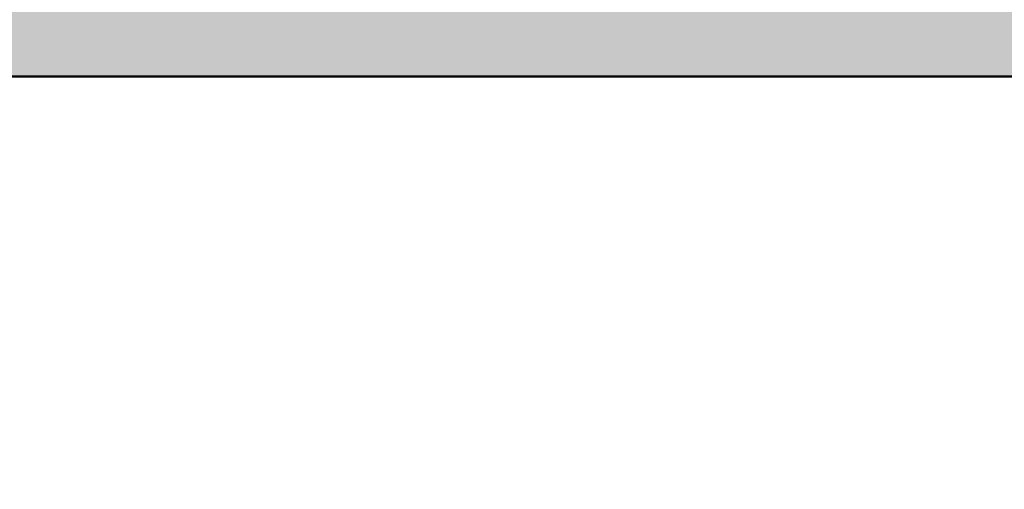
# Model space of a CAD drawing. Units: inches. Extents: x -7 to 1228, y -146 to 1091.
# Tile 65 of 88: x 656 to 745, y 531 to 573. Entities that reach past the tile are written whole.
import ezdxf

# ---------------------------------------------------------------- set-up
doc = ezdxf.new("R2010")
doc.units = ezdxf.units.IN
doc.layers.add('A-WALL', color=7, linetype='Continuous', lineweight=50)
doc.layers.add('A-WALL-PATT', color=251, linetype='Continuous', lineweight=13)

msp = doc.modelspace()

# ---------------------------------------------------------------- hatches: boundary and pattern name
at = {"layer": 'A-WALL-PATT'}
h = msp.add_hatch(color=256, dxfattribs=at)
h.dxf.hatch_style = 1
h.paths.add_polyline_path([(69, 568), (60, 568), (60, 493), (63.289, 493), (69, 493)])
h.paths.add_polyline_path([(69, 662.405), (60, 662.405), (60, 586), (69, 586)], flags=17)
h.paths.add_polyline_path([(69, 723), (184, 723), (184, 734), (179, 734), (179, 728), (69, 728), (69, 741.623), (60, 741.623), (60, 698.405), (69, 698.405)], flags=17)
h.paths.add_polyline_path([(69, 782), (231, 782), (231, 728), (231, 723), (231, 586), (236, 586), (236, 787), (69, 787), (69, 800.126), (60, 800.126), (60, 765.623), (69, 765.623)])
h.paths.add_polyline_path([(184, 842), (189, 842), (189, 848), (173, 848), (173, 842), (179, 842), (179, 787), (184, 787)])
h.paths.add_polyline_path([(118.22, 69), (69, 69), (69, 60), (118.22, 60)])
h.paths.add_polyline_path([(227, 69), (154.22, 69), (154.22, 60), (227, 60)])
h.paths.add_polyline_path([(236, 60), (232.711, 60), (227, 60), (227, 36), (236, 36)])
h.paths.add_polyline_path([(389, 60), (380, 60), (380, 36), (389, 36)])
h.paths.add_polyline_path([(384, 181), (380, 181), (380, 115), (380, 78), (384, 78)])
h.paths.add_polyline_path([(380, 115), (334.547, 115), (334.547, 109), (380, 109)])
h.paths.add_polyline_path([(274.547, 115), (236, 115), (236, 201), (232.711, 201), (231, 201), (231, 78), (236, 78), (236, 109), (274.547, 109)])
h.paths.add_polyline_path([(69, 123), (60, 123), (60, 78), (69, 78)])
h.paths.add_polyline_path([(69, 201), (60, 201), (60, 159), (69, 159)])
h.paths.add_polyline_path([(143, 219), (69, 219), (69, 213), (143, 213)], flags=17)
h.paths.add_polyline_path([(189, 219), (184, 219), (184, 274), (231, 274), (231, 219), (236, 219), (236, 279), (184, 279), (184, 297), (179, 297), (179, 279), (69, 279), (69, 290.912), (60, 290.912), (60, 262.179), (69, 262.179), (69, 274), (179, 274), (179, 219), (173, 219), (173, 213), (189, 213)])
h.paths.add_polyline_path([(69, 238.179), (60, 238.179), (60, 219), (69, 219)], flags=17)
h.paths.add_polyline_path([(69, 333), (60, 333), (60, 314.912), (69, 314.912), (69, 316.965)])
h.paths.add_polyline_path([(190, 338), (184, 338), (69, 338), (69, 333), (179, 333), (179, 327), (184, 327), (184, 333.021), (190, 333.046)])
h.paths.add_polyline_path([(69, 386.806), (60, 386.806), (60, 351), (69, 351)])
h.paths.add_polyline_path([(69, 475), (60, 475), (60, 422.806), (69, 422.806)])
h.paths.add_polyline_path([(236, 475), (231, 475), (231, 351.238), (236, 351.238)])
h.paths.add_polyline_path([(384, 475), (380, 475), (380, 362), (384, 362)])
h.paths.add_polyline_path([(547, 307), (439, 307), (439, 356), (445, 356), (445, 362), (433, 362), (433, 307), (380, 307), (380, 244), (380, 241), (384, 241), (384, 301), (433, 301), (433, 277), (439, 277), (439, 301), (547, 301)])
h.paths.add_polyline_path([(547, 241), (439, 241), (439, 247), (433, 247), (433, 235), (547, 235)])
h.paths.add_polyline_path([(450, 69), (440.286, 69), (424.889, 69), (389, 69), (389, 60), (450, 60)])
h.paths.add_polyline_path([(547, 69), (486, 69), (486, 60), (547, 60)])
h.paths.add_polyline_path([(556, 148.268), (547, 148.268), (547, 78), (556, 78)])
h.paths.add_polyline_path([(556, 223), (547, 223), (547, 195), (547, 184.268), (556, 184.268)])
h.paths.add_polyline_path([(556, 311.192), (547, 311.192), (547, 273.075), (556, 273.075)])
h.paths.add_polyline_path([(556, 344), (552.711, 344), (547, 344), (547, 335.192), (556, 335.192)])
h.paths.add_polyline_path([(556, 249.075), (547, 249.075), (547, 241), (556, 241)])
h.paths.add_polyline_path([(547, 362), (475, 362), (475, 356), (547, 356)], flags=0)
h.paths.add_polyline_path([(556, 399.621), (547, 399.621), (547, 362), (556, 362)])
h.paths.add_polyline_path([(556, 475), (547, 475), (547, 435.621), (556, 435.621)])
h.paths.add_polyline_path([(547, 493), (389, 493), (389, 487), (547, 487)])
h.paths.add_polyline_path([(380, 493), (278, 493), (278, 487), (380, 487)])
h.paths.add_polyline_path([(227, 493), (69, 493), (69, 487), (227, 487)])
h.paths.add_polyline_path([(643, 122.445), (634, 122.445), (634, 78), (643, 78)])
h.paths.add_polyline_path([(702.5, 69), (692.786, 69), (677.389, 69), (643, 69), (643, 60), (702.5, 60)])
h.paths.add_polyline_path([(798, 69), (738.5, 69), (738.5, 60), (798, 60)])
h.paths.add_polyline_path([(807, 60), (803.711, 60), (798, 60), (798, 36), (807, 36)])
h.paths.add_polyline_path([(807, 109), (846.751, 109), (846.751, 115), (807, 115), (807, 159), (802, 159), (802, 78), (807, 78)])
h.paths.add_polyline_path([(807, 201), (802, 201), (802, 195), (807, 195)])
h.paths.add_polyline_path([(643, 201), (634, 201), (634, 158.445), (643, 158.445)])
h.paths.add_polyline_path([(756, 225), (751, 225), (751, 219), (643, 219), (643, 213), (756, 213)])
h.paths.add_polyline_path([(643, 240.848), (634, 240.848), (634, 219), (643, 219)])
h.paths.add_polyline_path([(643, 274), (643, 288.629), (634, 288.629), (634, 264.848), (643, 264.848)])
h.paths.add_polyline_path([(802, 279), (756, 279), (756, 297), (751, 297), (751, 279), (643, 279), (643, 274), (751, 274), (751, 255), (756, 255), (756, 274), (802, 274)])
h.paths.add_polyline_path([(807, 333), (803.711, 333), (802, 333), (802, 279), (802, 274), (802, 219), (807, 219)])
h.paths.add_polyline_path([(956, 182), (951, 182), (951, 115), (906.751, 115), (906.751, 109), (951, 109), (951, 78), (956, 78)])
h.paths.add_polyline_path([(960, 60), (951, 60), (951, 36), (960, 36)])
h.paths.add_polyline_path([(1021, 69), (1005.781, 69), (960, 69), (960, 60), (1021, 60)])
h.paths.add_polyline_path([(956, 224), (951, 224), (951, 218), (956, 218)])
h.paths.add_polyline_path([(956, 302), (1004, 302), (1004, 278), (1010, 278), (1010, 302), (1118, 302), (1118, 290.809), (1127, 290.809), (1127, 326.968), (1118, 326.968), (1118, 320.966), (1118, 307), (1010, 307), (1010, 356), (1016, 356), (1016, 362), (1004, 362), (1004, 307), (951, 307), (951, 244), (951, 242), (954.289, 242), (956, 242)])
h.paths.add_polyline_path([(643, 333), (634, 333), (634, 312.629), (643, 312.629), (643, 316.965)])
h.paths.add_polyline_path([(756, 338), (643, 338), (643, 333), (751, 333), (751, 327), (756, 327)])
h.paths.add_polyline_path([(643, 388), (634, 388), (634, 351), (643, 351)])
h.paths.add_polyline_path([(807, 357), (802, 357), (802, 351), (807, 351)])
h.paths.add_polyline_path([(807, 475), (802, 475), (802, 393), (807, 393)])
h.paths.add_polyline_path([(643, 475), (634, 475), (634, 424), (643, 424)])
h.paths.add_polyline_path([(798, 493), (643, 493), (643, 487), (798, 487)])
h.paths.add_polyline_path([(634, 493), (556, 493), (556, 487), (634, 487)])
h.paths.add_polyline_path([(813, 493), (807, 493), (807, 487), (813, 487)])
h.paths.add_polyline_path([(951, 493), (849, 493), (849, 487), (951, 487)])
h.paths.add_polyline_path([(956, 484), (951, 484), (951, 374), (956, 374)])
h.paths.add_polyline_path([(1109, 493), (969, 493), (969, 487), (1109, 487)])
h.paths.add_polyline_path([(1127, 484), (1118, 484), (1118, 450.641), (1127, 450.641)])
h.paths.add_polyline_path([(1127, 414.641), (1118, 414.641), (1118, 365), (1127, 365)])
h.paths.add_polyline_path([(1109, 362), (1046, 362), (1046, 356), (1109, 356)], flags=17)
h.paths.add_polyline_path([(1127, 356), (1123.454, 356), (1118, 356), (1118, 350.968), (1127, 350.968)], flags=0)
h.paths.add_polyline_path([(1127, 266.809), (1118, 266.809), (1118, 262.361), (1118, 242), (1127, 242)], flags=17)
h.paths.add_polyline_path([(1118, 242), (1010, 242), (1010, 248), (1004, 248), (1004, 237), (1118, 237)])
h.paths.add_polyline_path([(1127, 224), (1118, 224), (1118, 170), (1127, 170)])
h.paths.add_polyline_path([(1127, 134), (1118, 134), (1118, 78), (1127, 78)])
h.paths.add_polyline_path([(1118, 69), (1057, 69), (1057, 60), (1118, 60)])
h.paths.add_polyline_path([(227, 571.546), (227, 574), (69, 574), (69, 568), (227, 568)])
h.paths.add_polyline_path([(380, 571.546), (380, 574), (278, 574), (278, 568), (380, 568)])
h.paths.add_polyline_path([(242, 574), (236, 574), (236, 568), (242, 568)])
h.paths.add_polyline_path([(547, 571.546), (547, 574), (389, 574), (389, 568), (547, 568)])
h.paths.add_polyline_path([(384, 733), (380, 733), (380, 586), (384, 586)])
h.paths.add_polyline_path([(556, 646), (634, 646), (634, 655), (547, 655), (547, 586), (556, 586)])
h.paths.add_polyline_path([(634, 574), (556, 574), (556, 568), (634, 568)])
h.paths.add_polyline_path([(643, 655), (634, 655), (634, 586), (643, 586)])
h.paths.add_polyline_path([(798, 574), (643, 574), (643, 568), (798, 568)])
h.paths.add_polyline_path([(643, 663.854), (634, 663.854), (634, 655), (643, 655)])
h.paths.add_polyline_path([(556, 676.967), (547, 676.967), (547, 655), (556, 655)])
h.paths.add_polyline_path([(556, 733), (547, 733), (547, 712.967), (556, 712.967)])
h.paths.add_polyline_path([(643, 710), (634, 710), (634, 699.854), (643, 699.854)])
h.paths.add_polyline_path([(807, 668), (802, 668), (802, 586), (807, 586)])
h.paths.add_polyline_path([(951, 574), (849, 574), (849, 568), (951, 568)])
h.paths.add_polyline_path([(956, 691), (951, 691), (951, 577), (956, 577)])
h.paths.add_polyline_path([(1109, 574), (969, 574), (969, 568), (1109, 568)])
h.paths.add_polyline_path([(1127, 643.403), (1118, 643.403), (1118, 577), (1127, 577)])
h.paths.add_polyline_path([(1127, 568), (1123.454, 568), (1118, 568), (1118, 493), (1127, 493)])
h.paths.add_polyline_path([(1127, 733), (1118, 733), (1118, 679.403), (1127, 679.403)])
h.paths.add_polyline_path([(1127, 777.348), (1118, 777.348), (1118, 770.035), (1118, 751), (1127, 751)], flags=17)
h.paths.add_polyline_path([(1118, 751), (1010, 751), (1010, 757), (1004, 757), (1004, 745), (1118, 745)])
h.paths.add_polyline_path([(956, 811), (1004, 811), (1004, 787), (1010, 787), (1010, 811), (1017.874, 811), (1017.874, 811.627, -0.414214), (1018.247, 812), (1031.978, 812, -0.414214), (1032.351, 811.627), (1032.351, 811), (1118, 811), (1118, 801.348), (1127, 801.348), (1127, 834.685), (1118, 834.685), (1118, 830.238), (1118, 817), (1010, 817), (1010, 866), (1016, 866), (1016, 872), (1004, 872), (1004, 817), (956, 817), (956, 866), (951, 866), (951, 751), (954.289, 751), (956, 751)])
h.paths.add_polyline_path([(1118, 872), (1046, 872), (1046, 866), (1118, 866)], flags=17)
h.paths.add_polyline_path([(1127, 924.711), (1118, 924.711), (1118, 884), (1127, 884)])
h.paths.add_polyline_path([(1127, 866), (1123.711, 866), (1118, 866), (1118, 858.685), (1127, 858.685)], flags=17)
h.paths.add_polyline_path([(956, 983), (951, 983), (951, 952), (807, 952), (807, 983), (802, 983), (802, 902), (807, 902), (807, 946), (951, 946), (951, 884), (956, 884)])
h.paths.add_polyline_path([(807, 842), (802, 842), (802, 787), (756, 787), (756, 806), (751, 806), (751, 787), (643, 787), (643, 782), (751, 782), (751, 764), (756, 764), (756, 782), (802, 782), (802, 728), (807, 728)])
h.paths.add_polyline_path([(756, 848), (643, 848), (643, 842), (751, 842), (751, 836), (756, 836)])
h.paths.add_polyline_path([(756, 734), (751, 734), (751, 728), (643, 728), (643, 723), (756, 723)])
h.paths.add_polyline_path([(643, 749.791), (634, 749.791), (634, 728), (637.289, 728), (643, 728)])
h.paths.add_polyline_path([(643, 805.405), (634, 805.405), (634, 773.791), (643, 773.791)])
h.paths.add_polyline_path([(643, 896.663), (634, 896.663), (634, 860), (637.289, 860), (643, 860)])
h.paths.add_polyline_path([(643, 842), (634, 842), (634, 829.405), (643, 829.405)])
h.paths.add_polyline_path([(643, 983), (634, 983), (634, 932.663), (643, 932.663)])
h.paths.add_polyline_path([(1127, 983), (1118, 983), (1118, 960.711), (1127, 960.711)])
h.paths.add_polyline_path([(1118, 1001), (1077.525, 1001), (1077.525, 992), (1118, 992)])
h.paths.add_polyline_path([(1041.525, 1001), (960, 1001), (960, 992), (1041.525, 992)])
h.paths.add_polyline_path([(960, 1025), (951, 1025), (951, 1001), (954.289, 1001), (960, 1001)])
h.paths.add_polyline_path([(807, 1025), (798, 1025), (798, 1001), (807, 1001)])
h.paths.add_polyline_path([(798, 1001), (738.5, 1001), (738.5, 992), (798, 992)])
h.paths.add_polyline_path([(702.5, 1001), (643, 1001), (643, 992), (702.5, 992)])
h.paths.add_polyline_path([(547, 1001), (499.113, 1001), (499.113, 992), (547, 992)])
h.paths.add_polyline_path([(463.113, 1001), (389, 1001), (389, 992), (463.113, 992)])
h.paths.add_polyline_path([(389, 1025), (380, 1025), (380, 1022), (380, 1001), (383.289, 1001), (389, 1001)])
h.paths.add_polyline_path([(236, 1025), (227, 1025), (227, 1001), (236, 1001)])
h.paths.add_polyline_path([(236, 983), (231, 983), (231, 860), (236, 860)])
h.paths.add_polyline_path([(274.547, 952), (236, 952), (236, 946), (274.547, 946)])
h.paths.add_polyline_path([(380, 952), (334.547, 952), (334.547, 946), (380, 946)])
h.paths.add_polyline_path([(384, 983), (380, 983), (380, 884), (383.289, 884), (384, 884)])
h.paths.add_polyline_path([(227, 1001), (155.012, 1001), (155.012, 992), (162.875, 992), (227, 992)])
h.paths.add_polyline_path([(119.012, 1001), (69, 1001), (69, 992), (119.012, 992)])
h.paths.add_polyline_path([(69, 983), (60, 983), (60, 922.987), (69, 922.987)])
h.paths.add_polyline_path([(69, 886.987), (60, 886.987), (60, 860), (63.289, 860), (69, 860)])
h.paths.add_polyline_path([(143, 848), (69, 848), (69, 842), (143, 842)])

# ---------------------------------------------------------------- linework, layer by layer
at = {"layer": 'A-WALL'}
msp.add_line((813, 568), (556, 568), dxfattribs=at)

doc.saveas('drawing.dxf')
